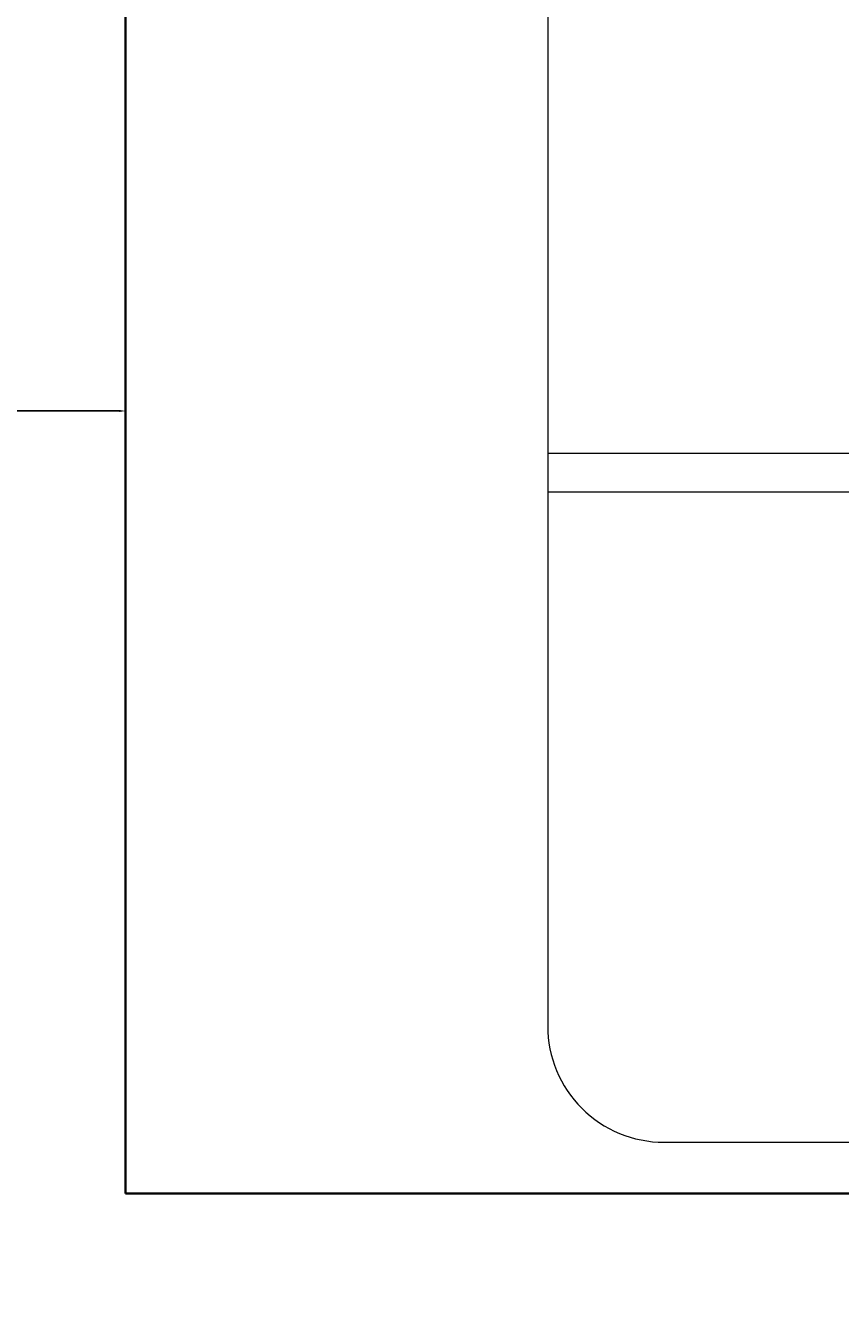
# Model space of a CAD drawing. Units: inches. Extents: x -61 to 1599, y -1316 to 257.
# Tile 114 of 204: x 85 to 109, y -10 to 27. Entities that reach past the tile are written whole.
import ezdxf

# ---------------------------------------------------------------- set-up
doc = ezdxf.new("R2010")
doc.units = ezdxf.units.IN
doc.header["$MEASUREMENT"] = 0
for name, color, linetype, lineweight in [('A-ANNO-DIMS', 2, 'Continuous', 18), ('FURNITURE', 83, 'Continuous', 18), ('WALLS', 4, 'Continuous', 35)]:
    doc.layers.add(name, color=color, linetype=linetype, lineweight=lineweight)
doc.styles.get("Standard").update_dxf_attribs({"font": 'arial.ttf'})
doc.dimstyles.get("Standard").update_dxf_attribs({"dimtxt": 0.18, "dimasz": 0.18, "dimexe": 0.18, "dimexo": 0.0625, "dimgap": 0.09, "dimtad": 0, "dimtih": 1, "dimtoh": 1, "dimdec": 0, "dimzin": 0, "dimdsep": 46, "dimlunit": 3, "dimtxsty": 'Standard', "dimcen": 0.09, "dimadec": 0, "dimazin": 0, "dimtfac": 1, "dimtdec": 0, "dimtofl": 0, "dimtmove": 0, "dimatfit": 3, "dimfxl": 1, "dimtolj": 1, "dimtzin": 0, "dimarcsym": 0})

# ---------------------------------------------------------------- blocks, each defined once
blk = doc.blocks.new('BED-DOUBLE')
for p, q in [((1.272, 20.467), (70.263, 20.467)), ((1.272, 19.317), (70.263, 19.317))]:
    blk.add_line(p, q)
blk.add_lwpolyline([(1.272, 88.537), (1.272, 3.449, 0.414214), (4.722, 0), (66.813, 0, 0.414214), (70.263, 3.449), (70.263, 88.537, 0.414214), (66.813, 91.987), (4.722, 91.987, 0.414214)], format="xyb", close=True)
blk = doc.blocks.new('*D645')
at = {"layer": 'A-ANNO-DIMS', "color": 0, "lineweight": -2, "transparency": 16777216}
for p, q in [((78.703, 28.303), (78.703, 15.745)), ((87.703, 28.303), (87.703, 15.745)), ((78.883, 15.925), (82.745, 15.925)), ((87.523, 15.925), (83.661, 15.925))]:
    blk.add_line(p, q, dxfattribs=at)
at = {"layer": 'A-ANNO-DIMS', "color": 0, "transparency": 16777216}
for points in [[(78.883, 15.955), (78.883, 15.895), (78.703, 15.925)], [(87.523, 15.955), (87.523, 15.895), (87.703, 15.925)]]:
    blk.add_solid(points, dxfattribs=at)
at = {"layer": 'DEFPOINTS', "color": 0, "transparency": 16777216}
for p in [(78.703, 28.365), (87.703, 28.365), (87.703, 15.925)]:
    blk.add_point(p, dxfattribs=at)
at = {"layer": 'A-ANNO-DIMS', "color": 0, "transparency": 16777216, "insert": (83.203, 15.925), "char_height": 0.18, "attachment_point": 5}
blk.add_mtext('\\A1;9 TYP.', dxfattribs=at)
blk = doc.blocks.new('*D687')
at = {"layer": 'A-ANNO-DIMS', "color": 0, "lineweight": -2, "transparency": 16777216}
for p, q in [((289.418, 181.677), (-61.077, 181.677)), ((-60.897, 181.497), (-60.897, -528.952)), ((-60.897, -1239.765), (-60.897, -529.316)), ((319.64, -1239.945), (-61.077, -1239.945))]:
    blk.add_line(p, q, dxfattribs=at)
at = {"layer": 'A-ANNO-DIMS', "color": 0, "transparency": 16777216}
for points in [[(-60.927, 181.497), (-60.867, 181.497), (-60.897, 181.677)], [(-60.927, -1239.765), (-60.867, -1239.765), (-60.897, -1239.945)]]:
    blk.add_solid(points, dxfattribs=at)
at = {"layer": 'DEFPOINTS', "color": 0, "transparency": 16777216}
for p in [(289.481, 181.677), (-60.897, -1239.945), (319.703, -1239.945)]:
    blk.add_point(p, dxfattribs=at)
at = {"layer": 'A-ANNO-DIMS', "color": 0, "transparency": 16777216, "insert": (-60.897, -529.134), "char_height": 0.18, "attachment_point": 5}
blk.add_mtext('\\A1;1421.6', dxfattribs=at)
blk = doc.blocks.new('*D700')
at = {"layer": 'A-ANNO-DIMS', "color": 0, "lineweight": -2, "transparency": 16777216}
for p, q in [((14.703, -616.882), (14.703, 257.457)), ((14.883, 257.277), (96.772, 257.277)), ((179.572, 257.277), (97.683, 257.277)), ((179.752, -616.882), (179.752, 257.457))]:
    blk.add_line(p, q, dxfattribs=at)
at = {"layer": 'A-ANNO-DIMS', "color": 0, "transparency": 16777216}
for points in [[(14.883, 257.307), (14.883, 257.247), (14.703, 257.277)], [(179.572, 257.307), (179.572, 257.247), (179.752, 257.277)]]:
    blk.add_solid(points, dxfattribs=at)
at = {"layer": 'DEFPOINTS', "color": 0, "transparency": 16777216}
for p in [(179.752, 257.277), (14.703, -616.945), (179.752, -616.945)]:
    blk.add_point(p, dxfattribs=at)
at = {"layer": 'A-ANNO-DIMS', "color": 0, "transparency": 16777216, "insert": (97.227, 257.277), "char_height": 0.18, "attachment_point": 5}
blk.add_mtext('\\A1;165.05', dxfattribs=at)

msp = doc.modelspace()

# ---------------------------------------------------------------- linework, layer by layer
at = {"layer": 'WALLS'}
for p, q in [((87.7028, 148.6771), (87.7028, -7.3229)), ((87.7028, -7.3229), (185.2611, -7.3229))]:
    msp.add_line(p, q, dxfattribs=at)

# ---------------------------------------------------------------- block references
at = {"layer": 'FURNITURE'}
msp.add_blockref('BED-DOUBLE', (98.977, -5.797), dxfattribs=at)

# ---------------------------------------------------------------- dimensions: what is measured, and where the dimension line sits
at = {"layer": 'A-ANNO-DIMS'}
dim = msp.add_linear_dim(base=(179.7521, 257.2771), p1=(14.7028, -616.9446), p2=(179.7521, -616.9446), dimstyle='Standard', override={"dimdec": 2, "dimlfac": 1, "dimrnd": 0, "dimzin": 0, "dimdsep": 46, "dimlunit": 2}, dxfattribs=at)
dim.commit()
dim.dimension.update_dxf_attribs({"geometry": '*D700', "text_midpoint": (97.2274, 257.2771)})
dim = msp.add_linear_dim(base=(-60.8972, -1239.9446), p1=(289.4807, 181.6771), p2=(319.7028, -1239.9446), angle=90, dimstyle='Standard', override={"dimdec": 1, "dimlfac": 1, "dimrnd": 0, "dimzin": 0, "dimdsep": 46, "dimlunit": 2}, dxfattribs=at)
dim.commit()
dim.dimension.update_dxf_attribs({"geometry": '*D687', "text_midpoint": (-60.8972, -529.1337)})
dim = msp.add_linear_dim(base=(87.7028, 15.9247), p1=(78.7028, 28.3651), p2=(87.7028, 28.3651), text='<> TYP.', dimstyle='Standard', override={"dimdec": 0, "dimlfac": 1, "dimrnd": 0, "dimzin": 0, "dimdsep": 46, "dimlunit": 2}, dxfattribs=at)
dim.commit()
dim.dimension.update_dxf_attribs({"geometry": '*D645', "text_midpoint": (83.2028, 15.9247)})

doc.saveas('drawing.dxf')
